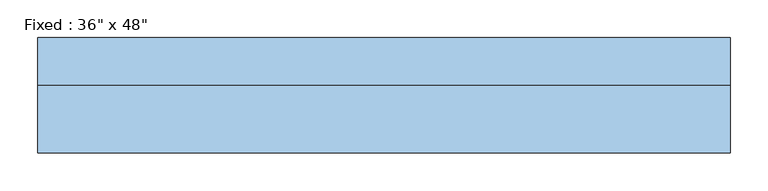
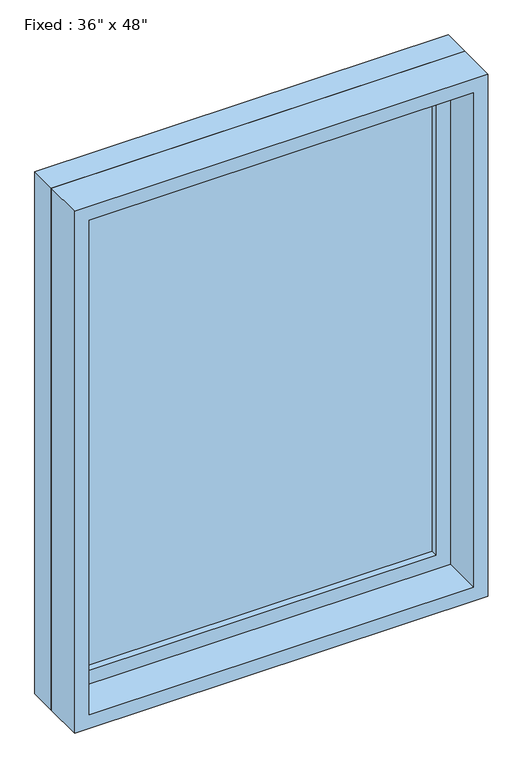
"""IFC4 building model written with IfcOpenShell, lengths in millimetres: window geometry."""

from ifc_helpers import new_model, si_unit, frame, origin, place, context, project, spatial, polyline, outline, extrude, source, transform, mapped, element, save


def window_d657a5cb(model_context):
    return source(origin(), model_context, "Body", "SweptSolid", [
        extrude(outline(polyline([(355.6, 28.575), (-431.8, 28.575), (-431.8, 41.275), (355.6, 41.275), (355.6, 28.575)])), frame((0.0, 0.0, 977.9), z_axis=(0.0, 0.0, 1.0), x_axis=(1.0, 0.0, 0.0)), (0.0, 0.0, 1.0), 1092.2),
        extrude(outline(polyline([(2114.55, -476.25), (933.45, -476.25), (933.45, 400.05), (2114.55, 400.05), (2114.55, -476.25)]), holes=[polyline([(2070.1, -431.8), (2070.1, 355.6), (977.9, 355.6), (977.9, -431.8), (2070.1, -431.8)])]), frame((0.0, 12.7, 0.0), z_axis=(0.0, 1.0, 0.0), x_axis=(0.0, 0.0, 1.0)), (0.0, 0.0, 1.0), 44.45),
        extrude(outline(polyline([(2133.6, -495.3), (914.4, -495.3), (914.4, 419.1), (2133.6, 419.1), (2133.6, -495.3)]), holes=[polyline([(2101.85, -463.55), (2101.85, 387.35), (946.15, 387.35), (946.15, -463.55), (2101.85, -463.55)])]), frame((0.0, -76.2, 0.0), z_axis=(0.0, 1.0, 0.0), x_axis=(0.0, 0.0, 1.0)), (0.0, 0.0, 1.0), 88.9),
        extrude(outline(polyline([(2133.6, 419.1), (2133.6, -495.3), (914.4, -495.3), (914.4, 419.1), (2133.6, 419.1)]), holes=[polyline([(2114.55, 400.05), (933.45, 400.05), (933.45, -476.25), (2114.55, -476.25), (2114.55, 400.05)])]), frame((0.0, 12.7, 0.0), z_axis=(0.0, 1.0, 0.0), x_axis=(0.0, 0.0, 1.0)), (0.0, 0.0, 1.0), 63.5),
    ])


if __name__ == "__main__":
    model = new_model("IFC4")
    model_context = context("Model", 3, world=origin())
    ifc_project = project(units=[si_unit("LENGTHUNIT", "METRE", prefix="MILLI")], contexts=[model_context])
    site = spatial("IfcSite", under=ifc_project)
    building = spatial("IfcBuilding", under=site)
    placement = place(None, origin())
    window_shape = window_d657a5cb(model_context)
    element("IfcWindow", 1, ObjectType="Fixed : 36\" x 48\"", at=placement, inside=building, context=model_context, shape_type="MappedRepresentation", body=[
        mapped(window_shape, transform((0.0, 0.0, 0.0), x_axis=(1.0, 0.0, 0.0), y_axis=(0.0, 1.0, 0.0), z_axis=(0.0, 0.0, 1.0))),
    ])
    save(model, "model.ifc")

# Revit data of these elements
# Type "Fixed : 36\" x 48\""
#   Type Mark = "1"
#   Construction Type Id = "GSP4R"
#   Assembly Code = "B2020100"
#   Analytic Construction = "1/8 in Pilkington single glazing"
#   Visual Light Transmittance = 0.9
#   Solar Heat Gain Coefficient = 0.78
#   Heat Transfer Coefficient (U) = 0.6496 BTU/(h·ft²·°F)
#   Height = 4' - 0"
#   Default Sill Height = 3' - 0"
#   Width = 3' - 0"
#   Window Inset = 0' - 0 3/4"
#   Define Thermal Properties by = 1
#   Glass Pane Material = Glass
#   Sash Material = Sash
#   Wall Closure = (empty or 0)
# Element 1 (IfcWindow, "Fixed : 36\" x 48\"")
#   Materials on its faces: "Sash", "Glass"
# Materials
#   "Glass": class "Glass", colour RGB 0 128 192, transparency 0.75, Description = "Soda Lime Glass", Cost = 0
#   "Sash": class "Wood", colour RGB 224 178 126, transparency 0
